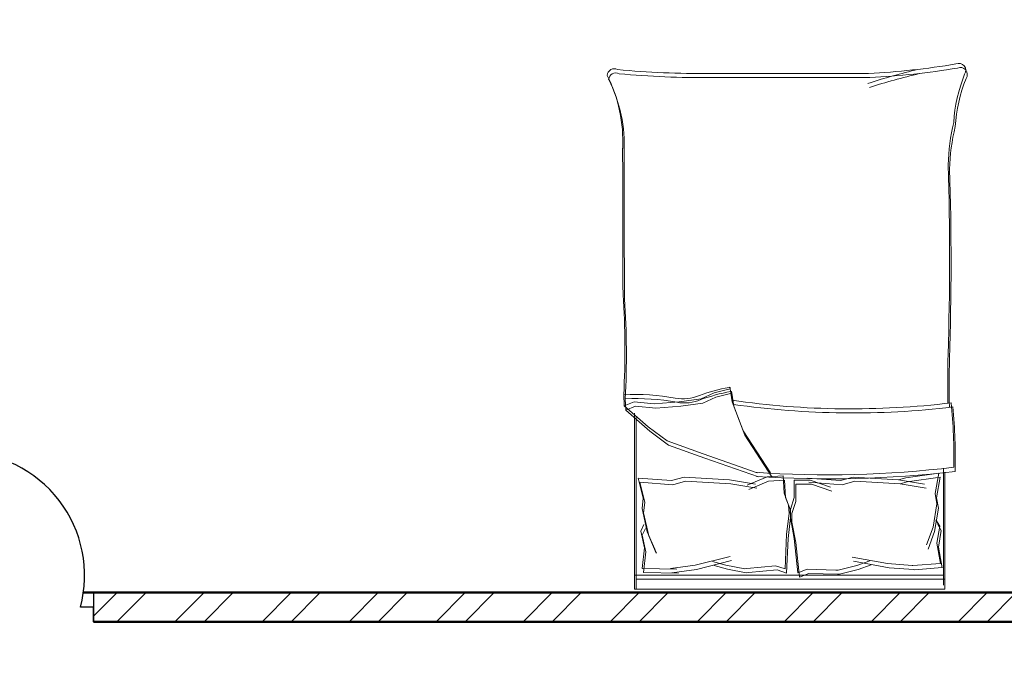
# Model space of a CAD drawing. Units: inches. Extents: x 963 to 2075, y 289 to 2657.
# Tile 56 of 98: x 1663 to 1815, y 1814 to 1915. Entities that reach past the tile are written whole.
import ezdxf

# ---------------------------------------------------------------- set-up
doc = ezdxf.new("R2010")
doc.units = ezdxf.units.IN
for name, color, linetype, lineweight in [('A-DOOR', 4, 'Continuous', 25), ('A-FURN', 8, 'Continuous', 18), ('A-WALL', 7, 'Continuous', 50), ('A-WALL-PATT', 8, 'Continuous', 13)]:
    doc.layers.add(name, color=color, linetype=linetype, lineweight=lineweight)

# ---------------------------------------------------------------- blocks, each defined once
blk = doc.blocks.new('BED-DOUBLE')
for p, q in [((1236.76, 2450.75), (1254.87, 2450.75)), ((1236.76, 2450.75), (1254.87, 2450.75)), ((1253.34, 2450.75), (1253.34, 2402.96)), ((1253.34, 2450.75), (1253.34, 2402.96)), ((1254.87, 2450.75), (1254.87, 2402.73)), ((1236.12, 2450.52), (1254.23, 2450.52)), ((1236.12, 2450.52), (1254.23, 2450.52)), ((1237.61, 2444.71), (1236.89, 2449.81)), ((1236.89, 2449.81), (1240.07, 2449.23)), ((1237.61, 2444.71), (1236.89, 2449.81)), ((1236.89, 2449.81), (1240.07, 2449.23)), ((1238.25, 2444.94), (1237.53, 2450.04)), ((1237.53, 2450.04), (1240.71, 2449.46)), ((1238.25, 2444.94), (1237.53, 2450.04)), ((1237.53, 2450.04), (1240.71, 2449.46)), ((1240.07, 2449.23), (1241.66, 2449.52)), ((1240.07, 2449.23), (1241.66, 2449.52)), ((1240.71, 2449.46), (1242.3, 2449.75)), ((1240.71, 2449.46), (1242.3, 2449.75)), ((1241.66, 2449.52), (1245.28, 2448.94)), ((1241.66, 2449.52), (1245.28, 2448.94)), ((1242.3, 2449.75), (1245.92, 2449.17)), ((1242.3, 2449.75), (1245.92, 2449.17)), ((1245.13, 2449.96), (1244.12, 2449.38)), ((1245.13, 2449.96), (1244.12, 2449.38)), ((1245.77, 2450.18), (1244.76, 2449.61)), ((1245.77, 2450.18), (1244.76, 2449.61)), ((1247.74, 2449.52), (1245.13, 2449.96)), ((1247.74, 2449.52), (1245.13, 2449.96)), ((1248.37, 2449.75), (1245.77, 2450.18)), ((1248.37, 2449.75), (1245.77, 2450.18)), ((1245.92, 2449.17), (1248.66, 2448.16)), ((1245.92, 2449.17), (1248.66, 2448.16)), ((1250.92, 2450.1), (1247.74, 2449.52)), ((1250.92, 2450.1), (1247.74, 2449.52)), ((1251.56, 2450.33), (1248.37, 2449.75)), ((1251.56, 2450.33), (1248.37, 2449.75)), ((1250.89, 2450.1), (1251.22, 2445.82)), ((1250.89, 2450.1), (1251.22, 2445.82)), ((1251.53, 2450.32), (1251.86, 2446.04)), ((1251.53, 2450.32), (1251.86, 2446.04)), ((1252.7, 2450.52), (1252.7, 2402.73)), ((1252.7, 2450.52), (1252.7, 2402.73)), ((1239.24, 2447.84), (1238.58, 2443.81)), ((1239.24, 2447.84), (1238.58, 2443.81)), ((1245.28, 2448.94), (1248.02, 2447.93)), ((1245.28, 2448.94), (1248.02, 2447.93)), ((1238.6, 2447.61), (1237.94, 2443.58)), ((1238.6, 2447.61), (1237.94, 2443.58)), ((1237.94, 2443.58), (1237.61, 2444.71)), ((1237.94, 2443.58), (1237.61, 2444.71)), ((1238.58, 2443.81), (1238.25, 2444.94)), ((1238.58, 2443.81), (1238.25, 2444.94)), ((1251.21, 2445.71), (1250.92, 2441.89)), ((1251.21, 2445.71), (1250.92, 2441.89)), ((1251.22, 2445.82), (1251.21, 2445.71)), ((1251.22, 2445.82), (1251.21, 2445.71)), ((1251.84, 2445.94), (1251.56, 2442.11)), ((1251.84, 2445.94), (1251.56, 2442.11)), ((1251.86, 2446.04), (1251.84, 2445.94)), ((1251.86, 2446.04), (1251.84, 2445.94)), ((1237.94, 2443.58), (1237.51, 2436.57)), ((1237.94, 2443.58), (1237.51, 2436.57)), ((1238.58, 2443.81), (1238.15, 2436.8)), ((1238.58, 2443.81), (1238.15, 2436.8)), ((1250.92, 2441.89), (1249.9, 2436.39)), ((1250.92, 2441.89), (1249.9, 2436.39)), ((1251.56, 2442.11), (1250.54, 2436.62)), ((1251.56, 2442.11), (1250.54, 2436.62)), ((1174.99, 2438.93), (1174.99, 2414.32)), ((1174.99, 2438.93), (1174.99, 2414.32)), ((1175.63, 2439.16), (1175.63, 2414.55)), ((1175.63, 2439.16), (1175.63, 2414.55)), ((1250.48, 2439.14), (1251.21, 2437.12)), ((1250.48, 2439.14), (1251.21, 2437.12)), ((1251.12, 2439.37), (1251.84, 2437.34)), ((1251.12, 2439.37), (1251.84, 2437.34)), ((1251.21, 2437.12), (1251.93, 2434.22)), ((1251.21, 2437.12), (1251.93, 2434.23)), ((1251.84, 2437.34), (1252.57, 2434.45)), ((1251.84, 2437.34), (1252.57, 2434.45)), ((1237.51, 2436.57), (1238.06, 2434.61)), ((1237.51, 2436.57), (1238.06, 2434.61)), ((1238.15, 2436.8), (1238.7, 2434.84)), ((1238.15, 2436.8), (1238.7, 2434.84)), ((1238.06, 2434.61), (1237.66, 2429.48)), ((1238.06, 2434.61), (1237.66, 2429.48)), ((1238.7, 2434.84), (1238.3, 2429.71)), ((1238.7, 2434.84), (1238.3, 2429.71)), ((1251.93, 2434.23), (1251.93, 2433.9)), ((1251.93, 2434.22), (1251.93, 2433.9)), ((1252.57, 2434.13), (1252.42, 2429.69)), ((1252.57, 2434.13), (1252.42, 2429.69)), ((1252.57, 2434.45), (1252.57, 2434.13)), ((1252.57, 2434.45), (1252.57, 2434.13)), ((1237.97, 2429.89), (1239.06, 2433.04)), ((1237.97, 2429.89), (1239.06, 2433.04)), ((1238.61, 2430.12), (1239.7, 2433.26)), ((1238.61, 2430.12), (1239.7, 2433.26)), ((1251.93, 2433.9), (1251.78, 2429.46)), ((1251.93, 2433.9), (1251.78, 2429.46)), ((1237.97, 2427.43), (1237.97, 2429.89)), ((1237.97, 2427.43), (1237.97, 2429.89)), ((1238.61, 2427.66), (1238.61, 2430.12)), ((1238.61, 2427.66), (1238.61, 2430.12)), ((1251.78, 2429.46), (1252.36, 2428.01)), ((1251.78, 2429.46), (1252.36, 2428.01)), ((1252.42, 2429.69), (1253, 2428.24)), ((1252.42, 2429.69), (1253, 2428.24)), ((1252.36, 2428.01), (1247.01, 2427.43)), ((1252.36, 2428.01), (1247.01, 2427.43)), ((1253, 2428.24), (1247.65, 2427.66)), ((1253, 2428.24), (1247.65, 2427.66)), ((1240.65, 2427.43), (1237.97, 2427.43)), ((1240.65, 2427.43), (1237.97, 2427.43)), ((1241.29, 2427.66), (1238.61, 2427.66)), ((1241.29, 2427.66), (1238.61, 2427.66)), ((1241.86, 2426.56), (1240.02, 2425.86)), ((1241.86, 2426.56), (1240.02, 2425.86)), ((1242.53, 2426.86), (1240.65, 2427.43)), ((1242.53, 2426.86), (1240.65, 2427.43)), ((1242.49, 2426.79), (1240.66, 2426.09)), ((1242.49, 2426.79), (1240.66, 2426.09)), ((1243.17, 2427.08), (1241.29, 2427.66)), ((1243.17, 2427.08), (1241.29, 2427.66)), ((1243.15, 2426.64), (1241.86, 2426.56)), ((1243.15, 2426.64), (1241.86, 2426.56)), ((1243.79, 2426.87), (1242.49, 2426.79)), ((1243.79, 2426.87), (1242.49, 2426.79)), ((1243.83, 2426.86), (1242.53, 2426.86)), ((1243.83, 2426.86), (1242.53, 2426.86)), ((1246.37, 2426.26), (1243.15, 2426.64)), ((1246.37, 2426.26), (1243.15, 2426.64)), ((1244.47, 2427.08), (1243.17, 2427.08)), ((1244.47, 2427.08), (1243.17, 2427.08)), ((1247, 2426.49), (1243.79, 2426.87)), ((1247, 2426.49), (1243.79, 2426.87)), ((1247.01, 2427.43), (1243.83, 2426.86)), ((1247.01, 2427.43), (1243.83, 2426.86)), ((1247.65, 2427.66), (1244.47, 2427.08)), ((1247.65, 2427.66), (1244.47, 2427.08)), ((1252.38, 2426.25), (1247, 2426.49)), ((1252.38, 2426.25), (1247, 2426.49)), ((1240.02, 2425.86), (1237.34, 2425.7)), ((1240.02, 2425.86), (1237.34, 2425.7)), ((1237.34, 2425.7), (1237.49, 2423.24)), ((1237.34, 2425.7), (1237.49, 2423.24)), ((1240.66, 2426.09), (1237.98, 2425.93)), ((1240.66, 2426.09), (1237.98, 2425.93)), ((1237.98, 2425.93), (1238.13, 2423.47)), ((1237.98, 2425.93), (1238.13, 2423.47)), ((1251.74, 2426.02), (1246.37, 2426.26)), ((1251.74, 2426.02), (1246.37, 2426.26)), ((1251.25, 2424.54), (1251.74, 2426.02)), ((1251.25, 2424.54), (1251.74, 2426.02)), ((1251.89, 2424.77), (1252.38, 2426.25)), ((1251.89, 2424.77), (1252.38, 2426.25)), ((1236.85, 2423.74), (1230.36, 2419.55)), ((1236.85, 2423.74), (1230.36, 2419.55)), ((1237.49, 2423.96), (1231, 2419.77)), ((1237.49, 2423.96), (1231, 2419.77)), ((1238.13, 2423.47), (1239.42, 2420.4)), ((1238.13, 2423.47), (1239.42, 2420.4)), ((1251.68, 2420.11), (1251.25, 2424.54)), ((1251.68, 2420.11), (1251.25, 2424.54)), ((1252.31, 2420.34), (1251.89, 2424.77)), ((1252.31, 2420.34), (1251.89, 2424.77)), ((1234.56, 2413.58), (1237.49, 2421.92)), ((1234.56, 2413.58), (1237.49, 2421.92)), ((1237.49, 2423.24), (1238.78, 2420.17)), ((1237.49, 2423.24), (1238.78, 2420.17)), ((1233.92, 2413.35), (1236.85, 2421.69)), ((1233.92, 2413.35), (1236.85, 2421.69)), ((1238.6, 2421.43), (1237.94, 2417.4)), ((1238.6, 2421.43), (1237.94, 2417.4)), ((1239.24, 2421.66), (1238.58, 2417.63)), ((1239.24, 2421.66), (1238.58, 2417.63)), ((1252.33, 2420.02), (1252.31, 2420.34)), ((1252.33, 2420.02), (1252.31, 2420.34)), ((1230.36, 2419.55), (1225.87, 2417.84)), ((1230.36, 2419.55), (1225.87, 2417.84)), ((1231, 2419.77), (1226.51, 2418.07)), ((1231, 2419.77), (1226.51, 2418.07)), ((1251.15, 2416.86), (1251.7, 2419.79)), ((1251.15, 2416.86), (1251.7, 2419.79)), ((1251.7, 2419.79), (1251.68, 2420.11)), ((1251.7, 2419.79), (1251.68, 2420.11)), ((1251.79, 2417.09), (1252.33, 2420.02)), ((1251.79, 2417.09), (1252.33, 2420.02)), ((1225.87, 2417.84), (1223.86, 2417.53)), ((1225.87, 2417.84), (1223.86, 2417.53)), ((1223.86, 2417.53), (1224.47, 2415.05)), ((1223.86, 2417.53), (1224.47, 2415.05)), ((1226.51, 2418.07), (1224.49, 2417.76)), ((1226.51, 2418.07), (1224.49, 2417.76)), ((1224.49, 2417.76), (1225.11, 2415.28)), ((1224.49, 2417.76), (1225.11, 2415.28)), ((1237.94, 2417.4), (1237.51, 2410.39)), ((1237.94, 2417.4), (1237.51, 2410.39)), ((1238.58, 2417.63), (1238.15, 2410.62)), ((1238.58, 2417.63), (1238.15, 2410.62)), ((1251.16, 2412.08), (1249.81, 2417.5)), ((1251.16, 2412.08), (1249.81, 2417.5)), ((1251.8, 2412.31), (1250.45, 2417.73)), ((1251.8, 2412.31), (1250.45, 2417.73)), ((1250.56, 2414.79), (1251.15, 2416.86)), ((1250.56, 2414.79), (1251.15, 2416.86)), ((1251.2, 2415.02), (1251.79, 2417.09)), ((1251.2, 2415.02), (1251.79, 2417.09)), ((1224.47, 2415.05), (1225.4, 2413.04)), ((1224.47, 2415.05), (1225.4, 2413.04)), ((1225.11, 2415.28), (1226.04, 2413.27)), ((1225.11, 2415.28), (1226.04, 2413.27)), ((1225.4, 2413.04), (1225.87, 2409.63)), ((1225.4, 2413.04), (1225.87, 2409.63)), ((1226.04, 2413.27), (1226.51, 2409.86)), ((1226.04, 2413.27), (1226.51, 2409.86)), ((1231.9, 2407.77), (1233.92, 2413.35)), ((1231.9, 2407.78), (1233.92, 2413.35)), ((1232.54, 2408), (1234.56, 2413.58)), ((1232.54, 2408), (1234.56, 2413.58)), ((1251.69, 2408.28), (1251.16, 2412.08)), ((1251.69, 2408.28), (1251.16, 2412.08)), ((1252.33, 2408.51), (1251.8, 2412.31)), ((1252.33, 2408.51), (1251.8, 2412.31)), ((1225.87, 2409.63), (1226.18, 2405.76)), ((1225.87, 2409.63), (1226.18, 2405.76)), ((1226.51, 2409.86), (1226.82, 2405.99)), ((1226.51, 2409.86), (1226.82, 2405.99)), ((1237.51, 2410.39), (1238.06, 2408.43)), ((1237.51, 2410.39), (1238.06, 2408.43)), ((1238.15, 2410.62), (1238.7, 2408.66)), ((1238.15, 2410.62), (1238.7, 2408.66)), ((1238.06, 2408.43), (1237.66, 2403.3)), ((1238.06, 2408.43), (1237.66, 2403.3)), ((1238.7, 2408.66), (1238.3, 2403.52)), ((1238.7, 2408.66), (1238.3, 2403.52)), ((1251.68, 2403.88), (1251.77, 2409.29)), ((1251.68, 2403.88), (1251.77, 2409.28)), ((1251.77, 2409.29), (1251.69, 2408.28)), ((1251.77, 2409.28), (1251.69, 2408.28)), ((1252.31, 2404.11), (1252.41, 2409.51)), ((1252.31, 2404.11), (1252.41, 2409.51)), ((1252.41, 2409.51), (1252.33, 2408.51)), ((1252.41, 2409.51), (1252.33, 2408.51)), ((1229.74, 2404.83), (1231.9, 2407.78)), ((1229.74, 2404.83), (1231.9, 2407.77)), ((1230.38, 2405.06), (1232.54, 2408)), ((1230.38, 2405.06), (1232.54, 2408)), ((1226.18, 2405.76), (1225.87, 2402.66)), ((1226.18, 2405.76), (1225.87, 2402.66)), ((1226.82, 2405.99), (1226.51, 2402.89)), ((1226.82, 2405.99), (1226.51, 2402.89)), ((1227.13, 2401.36), (1230.38, 2405.06)), ((1227.13, 2401.36), (1230.38, 2405.06)), ((1245.98, 2404.69), (1248.65, 2405.87)), ((1245.98, 2404.69), (1248.65, 2405.87)), ((1246.61, 2404.91), (1249.29, 2406.1)), ((1246.61, 2404.91), (1249.29, 2406.09)), ((1226.49, 2401.13), (1229.74, 2404.83)), ((1226.49, 2401.13), (1229.74, 2404.83)), ((1237.66, 2403.3), (1240.8, 2404.07)), ((1237.66, 2403.3), (1240.8, 2404.07)), ((1238.3, 2403.52), (1241.44, 2404.3)), ((1238.3, 2403.52), (1241.44, 2404.3)), ((1240.8, 2404.07), (1242.4, 2403.88)), ((1240.8, 2404.07), (1242.4, 2403.88)), ((1241.44, 2404.3), (1243.04, 2404.11)), ((1241.44, 2404.3), (1243.04, 2404.11)), ((1242.4, 2403.88), (1245.98, 2404.69)), ((1242.4, 2403.88), (1245.98, 2404.69)), ((1243.04, 2404.11), (1246.61, 2404.91)), ((1243.04, 2404.11), (1246.61, 2404.91)), ((1245.89, 2403.67), (1244.85, 2404.18)), ((1245.89, 2403.67), (1244.85, 2404.18)), ((1246.53, 2403.89), (1245.49, 2404.41)), ((1246.53, 2403.89), (1245.49, 2404.41)), ((1248.46, 2404.26), (1245.89, 2403.67)), ((1248.46, 2404.26), (1245.89, 2403.67)), ((1249.1, 2404.49), (1246.53, 2403.89)), ((1249.1, 2404.49), (1246.53, 2403.89)), ((1251.68, 2403.88), (1248.46, 2404.26)), ((1251.68, 2403.88), (1248.46, 2404.26)), ((1252.31, 2404.11), (1249.1, 2404.49)), ((1252.31, 2404.11), (1249.1, 2404.49)), ((1225.87, 2402.66), (1226.49, 2401.13)), ((1225.87, 2402.66), (1226.49, 2401.13)), ((1226.51, 2402.89), (1227.13, 2401.36)), ((1226.51, 2402.89), (1227.13, 2401.36)), ((1254.23, 2402.73), (1227.62, 2402.73)), ((1254.23, 2402.73), (1227.62, 2402.73)), ((1254.87, 2402.96), (1228.26, 2402.96)), ((1254.87, 2402.96), (1228.26, 2402.96)), ((1254.87, 2402.73), (1254.23, 2402.73)), ((1224.74, 2401.05), (1226.49, 2401.13, 3.87)), ((1224.74, 2401.05), (1226.49, 2401.13, 3.87)), ((1225.38, 2401.28), (1227.13, 2401.36, 3.87)), ((1225.38, 2401.28), (1227.13, 2401.36, 3.87))]:
    blk.add_line(p, q)
for centre, radius, start, end in [((1174.51, 2452.91), 1.09, 56.1736, 203.4781), ((1174.51, 2452.91), 1.09, 56.1736, 203.4781), ((1175.15, 2453.14), 1.09, 56.1736, 203.4781), ((1175.15, 2453.14), 1.09, 56.1736, 203.4781), ((1183.96, 2475.65), 23.56, 247.9751, 266.652), ((1183.96, 2475.65), 23.56, 247.9751, 266.652), ((1184.6, 2475.88), 23.56, 247.9751, 266.652), ((1184.6, 2475.88), 23.56, 247.9751, 266.652), ((1053.4, 2432.57), 121.76, 2.9958, 9.4091), ((1053.4, 2432.57), 121.76, 2.9958, 9.4091), ((1054.03, 2432.8), 121.76, 2.9958, 9.4091), ((1054.03, 2432.8), 121.76, 2.9958, 9.4091), ((1190.36, 2481.12), 29.63, 256.0648, 268.9113), ((1190.36, 2481.12), 29.63, 256.0648, 268.9113), ((1234.78, 2369.06), 83.31, 88.7218, 95.604), ((1234.78, 2369.06), 83.31, 88.7218, 95.604), ((1072.82, 2432.86), 164.97, 356.0865, 6.7821), ((1072.82, 2432.86), 164.97, 356.0865, 6.7821), ((1189.72, 2480.89), 29.63, 256.0648, 268.9113), ((1189.72, 2480.89), 29.63, 256.0648, 268.9113), ((1203.62, 1969.17), 482.31, 88.2277, 91.7185), ((1203.62, 1969.17), 482.31, 88.2277, 91.7185), ((1204.26, 1969.4), 482.31, 88.2277, 91.7185), ((1204.26, 1969.4), 482.31, 88.2277, 91.7185), ((1223.06, 2621.3), 170.11, 268.4762, 271.0082), ((1223.06, 2621.3), 170.11, 268.4762, 271.0082), ((1223.7, 2621.53), 170.11, 268.4762, 271.0082), ((1223.7, 2621.53), 170.11, 268.4762, 271.0082), ((1097.92, 2436.24), 129.02, 351.7845, 6.9006), ((1097.92, 2436.24), 129.02, 351.7845, 6.9006), ((1234.14, 2368.83), 83.31, 88.7218, 95.604), ((1234.14, 2368.83), 83.31, 88.7218, 95.604), ((1098.56, 2436.47), 129.02, 351.7845, 6.9006), ((1098.56, 2436.47), 129.02, 351.7845, 6.9006), ((1072.18, 2432.64), 164.97, 356.0865, 6.7821), ((1072.18, 2432.64), 164.97, 356.0865, 6.7821), ((1277.94, 2471.22), 106.46, 193.3832, 197.7053), ((1277.94, 2471.22), 106.46, 193.3832, 197.7053), ((1278.58, 2471.44), 106.46, 193.3832, 197.7053), ((1278.58, 2471.44), 106.46, 193.3832, 197.7053), ((1223.79, 2417.36), 0.185, 70.2464, 181.1377), ((1223.79, 2417.36), 0.185, 70.2464, 181.1377), ((1252.75, 2422.84), 29.65, 190.6617, 199.8806), ((1252.75, 2422.84), 29.65, 190.6617, 199.8806), ((1224.43, 2417.59), 0.185, 70.2464, 181.1377), ((1224.43, 2417.59), 0.185, 70.2464, 181.1377), ((1253.39, 2423.07), 29.65, 190.6617, 199.8806), ((1253.39, 2423.07), 29.65, 190.6617, 199.8806), ((1041.96, 2412.84), 133.04, 354.4998, 0.6351), ((1041.96, 2412.84), 133.04, 354.4998, 0.6351), ((1042.6, 2413.07), 133.04, 354.4998, 0.6351), ((1042.6, 2413.07), 133.04, 354.4998, 0.6351), ((1219.17, 2410.25), 6.22, 348.6608, 23.7384), ((1219.17, 2410.25), 6.22, 348.6608, 23.7384), ((1219.81, 2410.48), 6.22, 348.6608, 23.7384), ((1219.81, 2410.48), 6.22, 348.6608, 23.7384), ((1260.89, 2402.67), 36.18, 169.8763, 182.5657), ((1260.89, 2402.67), 36.18, 169.8763, 182.5657), ((1261.53, 2402.9), 36.18, 169.8763, 182.5657), ((1261.53, 2402.9), 36.18, 169.8763, 182.5657), ((1185.57, 2377.84), 23.07, 87.4714, 116.4681), ((1185.57, 2377.84), 23.07, 87.4714, 116.4681), ((1186.21, 2378.07), 23.07, 87.4714, 116.4681), ((1186.21, 2378.07), 23.07, 87.4714, 116.4681), ((1186.41, 6962.74), 4561.86, 270.00217, 270.28689), ((1186.41, 6962.74), 4561.86, 270.00217, 270.28689), ((1187.05, 6962.97), 4561.86, 270.00217, 270.28689), ((1187.05, 6962.97), 4561.86, 270.00217, 270.28689), ((1217.92, 2271.73), 129.5, 86.9791, 93.8365), ((1217.92, 2271.73), 129.5, 86.9791, 93.8365), ((1218.56, 2271.96), 129.5, 86.9791, 93.8365), ((1218.56, 2271.96), 129.5, 86.9791, 93.8365), ((1175.36, 2399.58), 1.1, 152.6588, 266.02), ((1175.36, 2399.58), 1.1, 152.6588, 266.02), ((1176, 2399.81), 1.1, 152.6588, 266.02), ((1176, 2399.81), 1.1, 152.6588, 266.02)]:
    blk.add_arc(centre, radius, start, end)

msp = doc.modelspace()

# ---------------------------------------------------------------- hatches: boundary and pattern name
at = {"layer": 'A-WALL-PATT'}
h = msp.add_hatch(dxfattribs=at)
h.set_pattern_fill('ANSI32', color=256)
h.paths.add_polyline_path([(1910.42, 1929.42), (1910.42, 1963.51), (1905.92, 1963.51), (1905.92, 1929.42), (1845.92, 1929.42), (1845.92, 1993.37), (1843.67, 1993.37), (1841.42, 1993.37), (1841.42, 1951.16), (1841.42, 1924.92), (1853.42, 1924.92), (1853.42, 1913.07), (1857.92, 1913.07), (1857.92, 1924.92), (1910.42, 1924.92)])
h.paths.add_polyline_path([(1857.92, 1853.07), (1853.42, 1853.07), (1853.42, 1826.32), (1841.42, 1826.32), (1674.48, 1826.32), (1674.48, 1821.82), (1853.42, 1821.82), (1857.92, 1821.82)])
h.paths.add_polyline_path([(1857.92, 1821.82), (1853.42, 1821.82), (1853.42, 1807.79), (1857.92, 1807.79)])
h.paths.add_polyline_path([(1857.92, 1747.79), (1853.42, 1747.79), (1853.42, 1713.82), (1809.34, 1713.82), (1809.34, 1709.32), (1905.92, 1709.32), (1905.92, 1688.32), (1910.42, 1688.32), (1910.42, 1713.82), (1857.92, 1713.82)])
h.paths.add_polyline_path([(1830.92, 1542.82), (1837.43, 1542.82), (1837.43, 1545.07), (1837.43, 1547.32), (1823.42, 1547.32), (1823.42, 1545.07), (1823.42, 1542.82), (1826.42, 1542.82), (1826.42, 1482.82), (1742.42, 1482.82), (1742.42, 1505.39), (1737.92, 1505.39), (1737.92, 1478.32), (1830.92, 1478.32)])
h.paths.add_polyline_path([(1938.92, 1619.32), (1934.42, 1619.32), (1910.42, 1619.32), (1910.42, 1628.32), (1908.17, 1628.32), (1905.92, 1628.32), (1905.92, 1614.82), (1934.42, 1614.82), (1934.42, 1547.32), (1905.92, 1547.32), (1899.59, 1547.32), (1899.59, 1542.82), (1910.42, 1542.82), (1938.92, 1542.82)])
h.paths.add_polyline_path([(1803.68, 1547.32), (1773.92, 1547.32), (1773.92, 1709.32), (1777.76, 1709.32), (1777.76, 1713.82), (1701.92, 1713.82), (1701.92, 1697.8), (1706.42, 1697.8), (1706.42, 1709.32), (1769.42, 1709.32), (1769.42, 1662.82), (1706.42, 1662.82), (1706.42, 1674.38), (1701.92, 1674.38), (1701.92, 1662.82), (1675.67, 1662.82), (1675.67, 1658.32), (1769.42, 1658.32), (1769.42, 1547.32), (1729.17, 1547.32), (1729.17, 1542.82), (1737.92, 1542.82), (1737.92, 1529.39), (1742.42, 1529.39), (1742.42, 1542.82), (1803.68, 1542.82)])
h.paths.add_polyline_path([(1595.42, 1542.82), (1599.24, 1542.82), (1599.24, 1547.32), (1584.36, 1547.32), (1584.36, 1542.82), (1590.92, 1542.82), (1590.92, 1436.32), (1595.42, 1436.32), (1595.42, 1440.82)])
h.paths.add_polyline_path([(1693.17, 1547.32), (1649.42, 1547.32), (1649.42, 1658.32), (1652.1, 1658.32), (1652.1, 1660.57), (1652.1, 1662.82), (1649.42, 1662.82), (1649.42, 1680.94), (1647.17, 1680.94), (1644.92, 1680.94), (1644.92, 1547.32), (1622.42, 1547.32), (1622.42, 1545.07), (1622.42, 1542.82), (1649.42, 1542.82), (1679.42, 1542.82), (1679.42, 1529.85), (1681.67, 1529.85), (1683.92, 1529.85), (1683.92, 1542.82), (1693.17, 1542.82), (1693.17, 1545.07)])
h.paths.add_polyline_path([(1683.92, 1505.85), (1679.42, 1505.85), (1679.42, 1483.8), (1595.42, 1483.8), (1595.42, 1479.3), (1683.92, 1479.3)])
h.paths.add_polyline_path([(1402.99, 1547.32), (1376.42, 1547.32), (1376.42, 1675.89), (1374.17, 1675.89), (1371.92, 1675.89), (1371.92, 1662.82), (1368.88, 1662.82), (1368.88, 1658.32), (1371.92, 1658.32), (1371.92, 1547.32), (1335.46, 1547.32), (1335.46, 1542.82), (1337.42, 1542.82), (1337.42, 1526.73), (1341.92, 1526.73), (1341.92, 1542.82), (1371.92, 1542.82), (1402.99, 1542.82)])

# ---------------------------------------------------------------- linework, layer by layer
at = {"layer": 'A-DOOR'}
for p, q in [((1674.48, 1826.32), (1674.48, 1821.82)), ((1674.48, 1824.07), (1672.48, 1824.07)), ((1674.48, 1821.82), (1674.48, 1824.07))]:
    msp.add_line(p, q, dxfattribs=at)
msp.add_arc((1654.04, 1828.99), 19.08, 345.0651, 90, dxfattribs=at)
at = {"layer": 'A-WALL'}
for p, q in [((1672.94, 1826.32), (1841.42, 1826.32)), ((1674.48, 1821.82), (1853.42, 1821.82))]:
    msp.add_line(p, q, dxfattribs=at)

# ---------------------------------------------------------------- block references
at = {"layer": 'A-FURN', "rotation": 269.9999998331857}
msp.add_blockref('BED-DOUBLE', (-644.47, 3081.73), dxfattribs=at)

doc.saveas('drawing.dxf')
